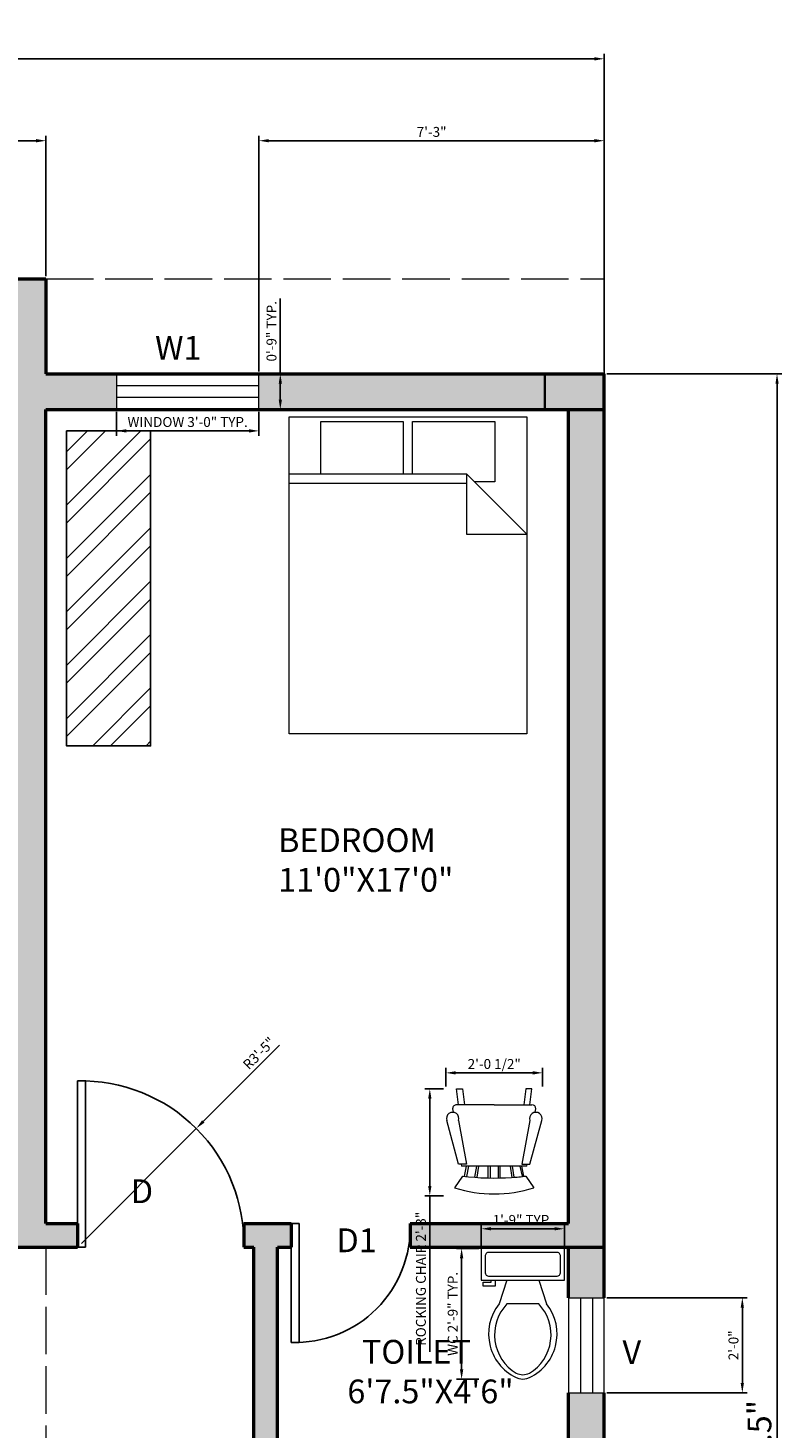
# Model space of a CAD drawing. Units: inches. Extents: x 5703 to 6226, y 10088 to 10813.
# Tile 5 of 5: x 6036 to 6226, y 10460 to 10813. Entities that reach past the tile are written whole.
import ezdxf

# ---------------------------------------------------------------- set-up
doc = ezdxf.new("R2010")
doc.units = ezdxf.units.IN
doc.linetypes.add('ACAD_ISO02W100', pattern=[15, 12, -3])
for name, color, linetype, lineweight in [('A-ANNO-DIMS', 2, 'Continuous', 18), ('A-ANNO-TEXT', 7, 'Continuous', 18), ('A-AREA-IDEN', 7, 'Continuous', 18), ('A-COLS', 7, 'Continuous', 35), ('A-COLS-PATT', 7, 'Continuous', 13), ('A-DOOR', 140, 'Continuous', 25), ('A-FLOR-CASE', 8, 'Continuous', 25), ('A-FLOR-CASE-PATT', 9, 'Continuous', 13), ('A-FLOR-FIXT', 8, 'Continuous', 18), ('A-FURN', 8, 'Continuous', 18), ('A-WALL', 7, 'Continuous', 50), ('A-WALL-PATT', 9, 'Continuous', 13)]:
    doc.layers.add(name, color=color, linetype=linetype, lineweight=lineweight)
for name, color, linetype, lineweight, true_color in [('A-GLAZ', 112, 'Continuous', 18, 0x1ce368), ('A-ROOF-OVHD', 30, 'ACAD_ISO02W100', 18, 0xf8991e), ('A-WALL-OVHD', 30, 'ACAD_ISO02W100', 18, 0xf8991e)]:
    doc.layers.add(name, color=color, linetype=linetype, lineweight=lineweight, true_color=true_color)
doc.styles.get("Standard").update_dxf_attribs({"font": 'arial.ttf'})
doc.dimstyles.new('ISO-25', dxfattribs={"dimtxt": 2.5, "dimasz": 2.5, "dimexe": 1.25, "dimexo": 0.625, "dimtad": 1, "dimlunit": 3, "dimtxsty": 'Standard', "dimcen": 2.5, "dimadec": 0, "dimazin": 0, "dimtfac": 1, "dimtmove": 0, "dimatfit": 3, "dimfxl": 1, "dimarcsym": 0})

# ---------------------------------------------------------------- blocks, each defined once
blk = doc.blocks.new('*D10')
at = {"layer": 'A-ANNO-DIMS', "color": 0, "lineweight": -2, "transparency": 16777216}
for p, q in [((5772.18, 10726.21), (5772.18, 10806.65)), ((5774.68, 10805.4), (6178.68, 10805.4)), ((6181.18, 10726.49), (6181.18, 10806.65))]:
    blk.add_line(p, q, dxfattribs=at)
at = {"layer": 'A-ANNO-DIMS', "color": 0, "transparency": 16777216}
for points in [[(5774.68, 10805.81), (5774.68, 10804.98), (5772.18, 10805.4)], [(6178.68, 10805.81), (6178.68, 10804.98), (6181.18, 10805.4)]]:
    blk.add_solid(points, dxfattribs=at)
at = {"layer": 'Defpoints', "color": 0, "transparency": 16777216}
for p in [(6181.18, 10805.4), (5772.18, 10725.59), (6181.18, 10725.87)]:
    blk.add_point(p, dxfattribs=at)
at = {"layer": 'A-ANNO-DIMS', "color": 0, "transparency": 16777216, "insert": (5976.68, 10809.09), "char_height": 6, "attachment_point": 5}
blk.add_mtext('34\'-0.99"', dxfattribs=at)
blk = doc.blocks.new('*D11')
at = {"layer": 'A-ANNO-DIMS', "color": 0, "lineweight": -2, "transparency": 16777216}
for p, q in [((6181.8, 10725.87), (6226.04, 10725.87)), ((6224.79, 10723.37), (6224.79, 10180.87)), ((6181.8, 10178.37), (6226.04, 10178.37))]:
    blk.add_line(p, q, dxfattribs=at)
at = {"layer": 'A-ANNO-DIMS', "color": 0, "transparency": 16777216}
for points in [[(6224.38, 10723.37), (6225.21, 10723.37), (6224.79, 10725.87)], [(6224.38, 10180.87), (6225.21, 10180.87), (6224.79, 10178.37)]]:
    blk.add_solid(points, dxfattribs=at)
at = {"layer": 'Defpoints', "color": 0, "transparency": 16777216}
for p in [(6181.18, 10725.87), (6181.18, 10178.37), (6224.79, 10178.37)]:
    blk.add_point(p, dxfattribs=at)
at = {"layer": 'A-ANNO-DIMS', "color": 0, "transparency": 16777216, "insert": (6221.12, 10452.12), "char_height": 6, "width": 12.5074, "attachment_point": 5, "rotation": 90}
blk.add_mtext('45\'-7.5"', dxfattribs=at)
blk = doc.blocks.new('Bed - Queen')
for p, q in [((0, -80.00003), (0, 0)), ((0, 0), (59.99999, 0)), ((59.99999, 0), (59.99999, -80.00003)), ((7.99999, -1.2), (28.79998, -1.2)), ((7.99999, -14.4), (7.99999, -1.2)), ((28.79998, -1.2), (28.79998, -14.4)), ((31.19999, -1.2), (51.99999, -1.2)), ((31.19999, -14.4), (31.19999, -1.2)), ((51.99999, -1.2), (51.99999, -16.4)), ((0, -14.4), (44.8, -14.4)), ((44.8, -16.8), (0, -16.8)), ((59.99999, -29.6), (44.8, -14.4)), ((44.8, -14.4), (44.8, -29.6)), ((51.99999, -16.4), (46.79936, -16.4)), ((44.8, -29.6), (59.99999, -29.6)), ((59.99999, -80.00003), (0, -80.00003))]:
    blk.add_line(p, q)
blk = doc.blocks.new('Toilet - top')
for p, q in [((9.5, -6), (9.5, -2)), ((-10, -8.5), (-8, -8.5)), ((-10, -9.5), (-10, -8.5)), ((-7, -9.5), (-10, -9.5)), ((-8, -8.5), (-8, -8)), ((-7, -8), (-7, -9.5)), ((-4, -8), (-6, -14)), ((4, -8), (6, -14)), ((4, -14), (-4, -14))]:
    blk.add_line(p, q)
blk.add_lwpolyline([(10.5, -8), (10.5, 0), (-10.5, 0), (-10.5, -8)], close=True)
for points in [[(-9.5, -2), (-9.5, -6)], [(8.5, -1), (-8.5, -1)], [(-8.5, -7), (8.5, -7)]]:
    blk.add_lwpolyline(points)
for centre, radius, start, end in [((-8.62, -1.88), 0.884, 81.8699, 188.1301), ((8.62, -1.88), 0.884, 351.8699, 98.1301), ((-8.62, -6.12), 0.884, 171.8699, 278.1301), ((8.62, -6.12), 0.884, 261.8699, 8.1301), ((3.52, -21.58), 12.17, 141.4691, 247.9714), ((4.2, -21.82), 11.33, 136.3677, 238.9468), ((-3.52, -21.58), 12.17, 292.0284, 38.5307), ((-4.2, -21.82), 11.33, 301.053, 43.6321), ((0, -27.88), 4, 245.7318, 294.2682), ((0, -29), 4, 254.8605, 285.1395)]:
    blk.add_arc(centre, radius, start, end)
blk = doc.blocks.new('Chair - Rocking')
for p, q in [((-8, -4.5), (-10, -1.5)), ((8, -4.5), (10, -1.5)), ((-8.23428, -6.99939), (-8.3093, -7.47958)), ((-8.23041, -7), (8.23915, -7)), ((-7.5, -4.5), (-7, -7)), ((-6.5, -7), (-7.02225, -4.43)), ((-4.5, -7), (-4.96674, -4.19951)), ((-4, -7), (-4.40532, -4.16272)), ((-1.5, -4.05012), (-1.5, -7)), ((-1, -7), (-1, -4.05012)), ((1, -7), (1, -4.04655)), ((1.5, -4.05012), (1.5, -7)), ((4, -7), (4.40187, -4.18694)), ((4.5, -7), (4.96761, -4.19437)), ((6.5, -7), (7, -4.4057)), ((7.5, -4.5), (7, -7)), ((8.31071, -7.48854), (8.23449, -7.00073)), ((-9, -7.5), (-12, -18.49999)), ((-7, -7.5), (-9, -7.5)), ((-9, -18.49999), (-7, -7.5)), ((7, -7.5), (9, -7.5)), ((9, -18.49999), (7, -7.5)), ((9, -7.5), (12, -18.49999)), ((-10.36644, -20.64523), (-10.5, -21.49999)), ((10.5, -21.49999), (10.3575, -20.58798)), ((-9, -22.49999), (-9.5, -26.49999)), ((0, -22.49999), (-9.5, -22.49999)), ((-8, -26.49999), (-7.5, -22.49999)), ((0, -22.49999), (9.5, -22.49999)), ((8, -26.49999), (7.5, -22.49999)), ((9, -22.49999), (9.5, -26.49999)), ((-9.5, -26.49999), (-8, -26.49999)), ((9.5, -26.49999), (8, -26.49999))]:
    blk.add_line(p, q)
for centre, radius, start, end in [((0, -34.08333), 34.08333, 72.93847, 107.0615), ((0, -68.25004), 64.25, 93.92211, 97.15267), ((0, -68.25004), 64.25, 82.84733, 93.92211), ((-10.5, -18.99999), 1.58114, 161.5651, 18.43495), ((10.5, -18.99999), 1.58114, 161.5651, 18.43495), ((-9.5, -21.49999), 1, 180, 270), ((9.5, -21.49999), 1, 270, 0)]:
    blk.add_arc(centre, radius, start, end)
blk = doc.blocks.new('WIN-36x9')
for p, q in [((0, 9), (0, 0)), ((36, 9), (0, 9)), ((36, 0), (36, 9)), ((36, 6), (0, 6)), ((36, 3), (0, 3)), ((0, 0), (36, 0))]:
    blk.add_line(p, q)
blk = doc.blocks.new('DOOR-SWING-30')
for p, q in [((0, 30.02), (0, 0.02)), ((2, 30.02), (0, 30.02)), ((2, 0.02), (2, 30.02)), ((0, 0.02), (2, 0.02))]:
    blk.add_line(p, q)
blk.add_arc((1, 29.02), 29.02, 268.0251, 1.9749)
blk = doc.blocks.new('*D20')
at = {"layer": 'A-ANNO-DIMS', "color": 0, "lineweight": -2, "transparency": 16777216}
for p, q in [((6149.48, 10505.1), (6143.9, 10505.1)), ((6145.15, 10474.55), (6145.15, 10502.6)), ((6149.48, 10472.05), (6143.9, 10472.05))]:
    blk.add_line(p, q, dxfattribs=at)
at = {"layer": 'A-ANNO-DIMS', "color": 0, "transparency": 16777216}
for points in [[(6144.73, 10502.6), (6145.57, 10502.6), (6145.15, 10505.1)], [(6144.73, 10474.55), (6145.57, 10474.55), (6145.15, 10472.05)]]:
    blk.add_solid(points, dxfattribs=at)
at = {"layer": 'Defpoints', "color": 0, "transparency": 16777216}
for p in [(6145.15, 10505.1), (6150.11, 10505.1), (6150.11, 10472.05)]:
    blk.add_point(p, dxfattribs=at)
at = {"layer": 'A-ANNO-DIMS', "color": 0, "transparency": 16777216, "insert": (6143.23, 10488.57), "char_height": 2.5, "attachment_point": 5, "rotation": 90}
blk.add_mtext('WC 2\'-9" TYP.', dxfattribs=at)
blk = doc.blocks.new('*D21')
at = {"layer": 'A-ANNO-DIMS', "color": 0, "lineweight": -2, "transparency": 16777216}
for p, q in [((6150.11, 10505.72), (6150.11, 10511.3)), ((6171.11, 10505.72), (6171.11, 10511.3)), ((6152.61, 10510.05), (6168.61, 10510.05))]:
    blk.add_line(p, q, dxfattribs=at)
at = {"layer": 'A-ANNO-DIMS', "color": 0, "transparency": 16777216}
for points in [[(6152.61, 10510.47), (6152.61, 10509.64), (6150.11, 10510.05)], [(6168.61, 10510.47), (6168.61, 10509.64), (6171.11, 10510.05)]]:
    blk.add_solid(points, dxfattribs=at)
at = {"layer": 'Defpoints', "color": 0, "transparency": 16777216}
for p in [(6171.11, 10510.05), (6150.11, 10505.1), (6171.11, 10505.1)]:
    blk.add_point(p, dxfattribs=at)
at = {"layer": 'A-ANNO-DIMS', "color": 0, "transparency": 16777216, "insert": (6160.61, 10511.96), "char_height": 2.5, "attachment_point": 5}
blk.add_mtext('1\'-9" TYP.', dxfattribs=at)
blk = doc.blocks.new('*D22')
at = {"layer": 'A-ANNO-DIMS', "color": 0, "lineweight": -2, "transparency": 16777216}
for p, q in [((6057.98, 10716.24), (6057.98, 10710.22)), ((6093.98, 10716.24), (6093.98, 10710.22)), ((6060.48, 10711.47), (6091.48, 10711.47))]:
    blk.add_line(p, q, dxfattribs=at)
at = {"layer": 'A-ANNO-DIMS', "color": 0, "transparency": 16777216}
for points in [[(6060.48, 10711.89), (6060.48, 10711.05), (6057.98, 10711.47)], [(6091.48, 10711.89), (6091.48, 10711.05), (6093.98, 10711.47)]]:
    blk.add_solid(points, dxfattribs=at)
at = {"layer": 'Defpoints', "color": 0, "transparency": 16777216}
for p in [(6057.98, 10716.87), (6093.98, 10716.87), (6093.98, 10711.47)]:
    blk.add_point(p, dxfattribs=at)
at = {"layer": 'A-ANNO-DIMS', "color": 0, "transparency": 16777216, "insert": (6075.98, 10713.39), "char_height": 2.5, "attachment_point": 5}
blk.add_mtext('WINDOW 3\'-0" TYP.', dxfattribs=at)
blk = doc.blocks.new('*D23')
at = {"layer": 'A-ANNO-DIMS', "color": 0, "lineweight": -2, "transparency": 16777216}
for p, q in [((6099.38, 10725.87), (6099.38, 10744.86)), ((6094.61, 10725.87), (6100.63, 10725.87)), ((6099.38, 10719.37), (6099.38, 10723.37)), ((6094.61, 10716.87), (6100.63, 10716.87))]:
    blk.add_line(p, q, dxfattribs=at)
at = {"layer": 'A-ANNO-DIMS', "color": 0, "transparency": 16777216}
for points in [[(6098.97, 10723.37), (6099.8, 10723.37), (6099.38, 10725.87)], [(6098.97, 10719.37), (6099.8, 10719.37), (6099.38, 10716.87)]]:
    blk.add_solid(points, dxfattribs=at)
at = {"layer": 'Defpoints', "color": 0, "transparency": 16777216}
for p in [(6093.98, 10725.87), (6099.38, 10725.87), (6093.98, 10716.87)]:
    blk.add_point(p, dxfattribs=at)
at = {"layer": 'A-ANNO-DIMS', "color": 0, "transparency": 16777216, "insert": (6097.48, 10736.61), "char_height": 2.5, "attachment_point": 5, "rotation": 90}
blk.add_mtext('0\'-9" TYP.', dxfattribs=at)
blk = doc.blocks.new('*D34')
at = {"layer": 'A-ANNO-DIMS', "color": 0, "lineweight": -2, "transparency": 16777216}
for p, q in [((6140.55, 10545.36), (6135.87, 10545.36)), ((6137.12, 10542.86), (6137.12, 10520.86)), ((6140.55, 10518.36), (6135.87, 10518.36)), ((6137.12, 10518.36), (6137.12, 10478.99))]:
    blk.add_line(p, q, dxfattribs=at)
at = {"layer": 'A-ANNO-DIMS', "color": 0, "transparency": 16777216}
for points in [[(6136.71, 10542.86), (6137.54, 10542.86), (6137.12, 10545.36)], [(6136.71, 10520.86), (6137.54, 10520.86), (6137.12, 10518.36)]]:
    blk.add_solid(points, dxfattribs=at)
at = {"layer": 'Defpoints', "color": 0, "transparency": 16777216}
for p in [(6141.17, 10545.36), (6137.12, 10518.36), (6141.17, 10518.36)]:
    blk.add_point(p, dxfattribs=at)
at = {"layer": 'A-ANNO-DIMS', "color": 0, "transparency": 16777216, "insert": (6135.2, 10497.42), "char_height": 2.5, "attachment_point": 5, "rotation": 90}
blk.add_mtext('ROCKING CHAIR 2\'-3"', dxfattribs=at)
blk = doc.blocks.new('*D35')
at = {"layer": 'A-ANNO-DIMS', "color": 0, "lineweight": -2, "transparency": 16777216}
for p, q in [((6141.17, 10545.98), (6141.17, 10550.66)), ((6165.61, 10545.98), (6165.61, 10550.66)), ((6163.11, 10549.41), (6143.67, 10549.41))]:
    blk.add_line(p, q, dxfattribs=at)
at = {"layer": 'A-ANNO-DIMS', "color": 0, "transparency": 16777216}
for points in [[(6143.67, 10549.83), (6143.67, 10548.99), (6141.17, 10549.41)], [(6163.11, 10549.83), (6163.11, 10548.99), (6165.61, 10549.41)]]:
    blk.add_solid(points, dxfattribs=at)
at = {"layer": 'Defpoints', "color": 0, "transparency": 16777216}
for p in [(6141.17, 10549.41), (6141.17, 10545.36), (6165.61, 10545.36)]:
    blk.add_point(p, dxfattribs=at)
at = {"layer": 'A-ANNO-DIMS', "color": 0, "transparency": 16777216, "insert": (6153.39, 10551.33), "char_height": 2.5, "attachment_point": 5}
blk.add_mtext('2\'-0 1/2"', dxfattribs=at)
blk = doc.blocks.new('*D44')
at = {"layer": 'A-ANNO-DIMS', "color": 0, "lineweight": -2, "transparency": 16777216}
for p, q in [((5902.18, 10750.49), (5902.18, 10785.97)), ((5904.68, 10784.72), (6037.68, 10784.72)), ((6040.18, 10750.49), (6040.18, 10785.97))]:
    blk.add_line(p, q, dxfattribs=at)
at = {"layer": 'A-ANNO-DIMS', "color": 0, "transparency": 16777216}
for points in [[(5904.68, 10785.14), (5904.68, 10784.3), (5902.18, 10784.72)], [(6037.68, 10785.14), (6037.68, 10784.3), (6040.18, 10784.72)]]:
    blk.add_solid(points, dxfattribs=at)
at = {"layer": 'Defpoints', "color": 0, "transparency": 16777216}
for p in [(6040.18, 10784.72), (5902.18, 10749.87), (6040.18, 10749.87)]:
    blk.add_point(p, dxfattribs=at)
at = {"layer": 'A-ANNO-DIMS', "color": 0, "transparency": 16777216, "insert": (5971.18, 10786.62), "char_height": 2.5, "attachment_point": 5}
blk.add_mtext('11\'-6"', dxfattribs=at)
blk = doc.blocks.new('*D54')
at = {"layer": 'A-ANNO-DIMS', "color": 0, "lineweight": -2, "transparency": 16777216}
for p, q in [((6181.8, 10492.63), (6217.28, 10492.63)), ((6216.03, 10471.13), (6216.03, 10490.13)), ((6181.8, 10468.63), (6217.28, 10468.63))]:
    blk.add_line(p, q, dxfattribs=at)
at = {"layer": 'A-ANNO-DIMS', "color": 0, "transparency": 16777216}
for points in [[(6215.61, 10490.13), (6216.44, 10490.13), (6216.03, 10492.63)], [(6215.61, 10471.13), (6216.44, 10471.13), (6216.03, 10468.63)]]:
    blk.add_solid(points, dxfattribs=at)
at = {"layer": 'Defpoints', "color": 0, "transparency": 16777216}
for p in [(6181.18, 10492.63), (6216.03, 10492.63), (6181.18, 10468.63)]:
    blk.add_point(p, dxfattribs=at)
at = {"layer": 'A-ANNO-DIMS', "color": 0, "transparency": 16777216, "insert": (6214.12, 10480.63), "char_height": 2.5, "attachment_point": 5, "rotation": 90}
blk.add_mtext('2\'-0"', dxfattribs=at)
blk = doc.blocks.new('*D57')
at = {"layer": 'A-ANNO-DIMS', "color": 0, "lineweight": -2, "transparency": 16777216}
for p, q in [((6093.98, 10726.49), (6093.98, 10785.97)), ((6096.48, 10784.72), (6178.68, 10784.72)), ((6181.18, 10726.49), (6181.18, 10785.97))]:
    blk.add_line(p, q, dxfattribs=at)
at = {"layer": 'A-ANNO-DIMS', "color": 0, "transparency": 16777216}
for points in [[(6096.48, 10785.14), (6096.48, 10784.3), (6093.98, 10784.72)], [(6178.68, 10785.14), (6178.68, 10784.3), (6181.18, 10784.72)]]:
    blk.add_solid(points, dxfattribs=at)
at = {"layer": 'Defpoints', "color": 0, "transparency": 16777216}
for p in [(6181.18, 10784.72), (6093.98, 10725.87), (6181.18, 10725.87)]:
    blk.add_point(p, dxfattribs=at)
at = {"layer": 'A-ANNO-DIMS', "color": 0, "transparency": 16777216, "insert": (6137.58, 10786.62), "char_height": 2.5, "attachment_point": 5}
blk.add_mtext('7\'-3"', dxfattribs=at)
blk = doc.blocks.new('*D59')
at = {"layer": 'A-ANNO-DIMS', "color": 0, "lineweight": -2, "transparency": 16777216}
for p, q in [((6099.2, 10556.41), (6079.93, 10537.14)), ((6049.16, 10506.37), (6078.16, 10535.37))]:
    blk.add_line(p, q, dxfattribs=at)
at = {"layer": 'A-ANNO-DIMS', "color": 0, "transparency": 16777216}
blk.add_solid([(6079.63, 10537.43), (6080.22, 10536.84), (6078.16, 10535.37)], dxfattribs=at)
at = {"layer": 'Defpoints', "color": 0, "transparency": 16777216}
for p in [(6078.16, 10535.37), (6049.16, 10506.37)]:
    blk.add_point(p, dxfattribs=at)
at = {"layer": 'A-ANNO-DIMS', "color": 0, "transparency": 16777216, "insert": (6094.22, 10554.11), "char_height": 2.5, "attachment_point": 5, "rotation": 45.0005}
blk.add_mtext('R3\'-5"', dxfattribs=at)

msp = doc.modelspace()

# ---------------------------------------------------------------- hatches: boundary and pattern name
at = {"layer": 'A-COLS-PATT'}
h = msp.add_hatch(color=256, dxfattribs=at)
h.dxf.hatch_style = 1
h.paths.add_polyline_path([(5788.176, 10725.869), (5773.176, 10725.869), (5773.176, 10716.869), (5788.176, 10716.869)])
h.paths.add_polyline_path([(5782.176, 10516.684), (5773.176, 10516.684), (5773.176, 10497.849), (5782.176, 10497.849)])
h.paths.add_polyline_path([(5782.176, 10319.369), (5773.176, 10319.369), (5773.176, 10304.369), (5782.176, 10304.369)])
h.paths.add_polyline_path([(5960.955, 10313.369), (5953.525, 10313.369), (5953.525, 10304.369), (5960.955, 10304.369)])
h.paths.add_polyline_path([(6040.176, 10314.869), (6031.176, 10314.869), (6031.176, 10304.369), (6040.176, 10304.369)])
h.paths.add_polyline_path([(6181.176, 10198.545), (6172.176, 10198.545), (6172.176, 10178.369), (6181.176, 10178.369)])
h.paths.add_polyline_path([(6181.176, 10505.369), (6172.176, 10505.369), (6172.176, 10492.633), (6181.176, 10492.633)])
h.paths.add_polyline_path([(6181.176, 10725.869), (6166.176, 10725.869), (6166.176, 10716.869), (6181.176, 10716.869)])
at = {"layer": 'A-FLOR-CASE-PATT'}
h = msp.add_hatch(dxfattribs=at)
h.set_pattern_fill('ANSI32', color=256)
h.paths.add_polyline_path([(6066.642, 10711.473), (6045.414, 10711.473), (6045.414, 10631.936), (6066.642, 10631.936)])
at = {"layer": 'A-WALL-PATT'}
h = msp.add_hatch(color=256, dxfattribs=at)
h.dxf.hatch_style = 1
h.paths.add_polyline_path([(6057.982, 10725.869), (6040.176, 10725.869), (6040.176, 10749.869), (5999.271, 10749.869), (5999.271, 10740.869), (6031.176, 10740.869), (6031.176, 10716.869), (6031.176, 10511.369), (6013.525, 10511.369), (6013.525, 10505.369), (6048.161, 10505.369), (6048.161, 10511.369), (6040.176, 10511.369), (6040.176, 10716.869), (6057.982, 10716.869)])
h.paths.add_polyline_path([(6166.176, 10725.869), (6093.982, 10725.869), (6093.982, 10716.869), (6166.176, 10716.869)])
h.paths.add_polyline_path([(6181.176, 10716.869), (6172.176, 10716.869), (6172.176, 10511.369), (6132.161, 10511.369, -0.0172363), (6132.161, 10509.369), (6132.161, 10505.369), (6181.176, 10505.369)])
h.paths.add_polyline_path([(6181.176, 10468.633), (6172.176, 10468.633), (6172.176, 10451.369), (6098.676, 10451.369), (6098.676, 10505.369), (6102.161, 10505.369), (6102.161, 10511.369), (6090.161, 10511.369), (6090.161, 10507.369, -0.0121933), (6090.161, 10505.369), (6092.676, 10505.369), (6092.676, 10451.369), (6085.668, 10451.369), (6085.668, 10445.369), (6092.676, 10445.369), (6172.176, 10445.369), (6172.176, 10342.529), (6181.176, 10342.529)])
h.paths.add_polyline_path([(6181.176, 10282.529), (6172.176, 10282.529), (6172.176, 10253.369), (6092.676, 10253.369), (6092.676, 10247.369), (6094.176, 10247.369), (6094.176, 10238.954), (6100.176, 10238.954), (6100.176, 10247.369), (6172.176, 10247.369), (6172.176, 10234.545), (6181.176, 10234.545)])
h.paths.add_polyline_path([(6172.176, 10187.369), (6100.176, 10187.369), (6100.176, 10220.954), (6096.176, 10220.954, -0.0293864), (6094.176, 10220.954), (6094.176, 10178.369), (6172.176, 10178.369)])
h.paths.add_polyline_path([(6050.745, 10187.369), (6040.176, 10187.369), (6040.176, 10178.369), (6050.745, 10178.369)])
h.paths.add_polyline_path([(6040.176, 10187.369), (6031.176, 10187.369), (6031.176, 10178.369), (6040.176, 10178.369)])
h.paths.add_polyline_path([(6040.176, 10304.369), (6031.176, 10304.369), (6031.176, 10187.369), (6040.176, 10187.369)])
h.paths.add_polyline_path([(6040.176, 10393.328), (6031.176, 10393.328), (6031.176, 10314.869), (6040.176, 10314.869)])
h.paths.add_polyline_path([(6040.176, 10445.369), (6046.458, 10445.369), (6046.458, 10451.369), (6031.176, 10451.369), (6031.176, 10408.328), (6040.176, 10408.328)])
h.paths.add_polyline_path([(5911.176, 10584.869), (5845.666, 10584.869, -0.0172363), (5845.666, 10582.869), (5845.666, 10578.869), (5902.176, 10578.869), (5902.176, 10505.369), (5953.525, 10505.369), (5953.525, 10511.369), (5911.176, 10511.369)])
h.paths.add_polyline_path([(5902.176, 10511.369), (5782.176, 10511.369), (5782.176, 10505.369), (5902.176, 10505.369)])
h.paths.add_polyline_path([(5782.176, 10578.869), (5815.666, 10578.869), (5815.666, 10584.869), (5773.176, 10584.869), (5773.176, 10516.684), (5782.176, 10516.684)])
h.paths.add_polyline_path([(5782.176, 10497.849), (5773.176, 10497.849), (5773.176, 10438.429), (5782.176, 10438.429)])
h.paths.add_polyline_path([(5782.176, 10378.429), (5773.176, 10378.429), (5773.176, 10319.369), (5782.176, 10319.369)])
h.paths.add_polyline_path([(5824.846, 10313.369), (5782.176, 10313.369), (5782.176, 10304.369), (5824.846, 10304.369)])
h.paths.add_polyline_path([(5953.525, 10313.369), (5872.846, 10313.369), (5872.846, 10304.369), (5953.525, 10304.369)])

# ---------------------------------------------------------------- linework, layer by layer
at = {"layer": 'A-COLS'}
for p, q in [((6181.176, 10725.869), (6166.176, 10725.869)), ((6166.176, 10725.869), (6166.176, 10716.869))]:
    msp.add_line(p, q, dxfattribs=at)
at = {"layer": 'A-DOOR'}
for p, q in [((6048.161, 10505.369), (6048.161, 10547.369)), ((6048.161, 10547.369), (6050.161, 10547.369)), ((6050.161, 10547.369), (6050.161, 10505.369)), ((6102.161, 10511.369), (6102.161, 10511.369)), ((6050.161, 10505.369), (6048.161, 10505.369))]:
    msp.add_line(p, q, dxfattribs=at)
msp.add_arc((6049.161, 10506.369), 41.012, 358.60282, 91.39718, dxfattribs=at)
at = {"layer": 'A-FLOR-CASE'}
msp.add_lwpolyline([(6045.414, 10711.473), (6066.642, 10711.473), (6066.642, 10631.936), (6045.414, 10631.936)], close=True, dxfattribs=at)
at = {"layer": 'A-GLAZ'}
for p, q in [((6172.176, 10492.633), (6181.176, 10492.633)), ((6172.176, 10492.633), (6172.176, 10468.633)), ((6175.176, 10492.633), (6175.176, 10468.633)), ((6178.176, 10492.633), (6178.176, 10468.633)), ((6181.176, 10468.633), (6181.176, 10492.633)), ((6172.176, 10468.633), (6181.176, 10468.633)), ((6172.176, 10468.633), (6181.176, 10468.633))]:
    msp.add_line(p, q, dxfattribs=at)
at = {"layer": 'A-ROOF-OVHD'}
for p, q in [((6040.176, 10749.869), (6181.176, 10749.869)), ((6181.176, 10749.869), (6181.176, 10725.869))]:
    msp.add_line(p, q, dxfattribs=at)
at = {"layer": 'A-WALL'}
for p, q in [((5902.176, 10749.869), (6040.176, 10749.869)), ((6040.176, 10749.869), (6040.176, 10725.869)), ((6040.176, 10725.869), (6181.176, 10725.869)), ((6181.176, 10492.633), (6181.176, 10725.869)), ((6040.176, 10716.869), (6181.176, 10716.869)), ((6040.176, 10511.369), (6040.176, 10716.869)), ((6172.176, 10511.369), (6172.176, 10716.869)), ((6040.176, 10511.369), (6048.161, 10511.369)), ((6048.161, 10511.369), (6048.161, 10505.369)), ((6090.161, 10511.369), (6090.161, 10505.369)), ((6090.161, 10511.369), (6102.161, 10511.369)), ((6102.161, 10511.369), (6102.161, 10505.369)), ((6132.161, 10511.369), (6132.161, 10505.369)), ((6132.161, 10511.369), (6172.176, 10511.369)), ((6013.525, 10505.369), (6048.161, 10505.369)), ((6090.161, 10505.369), (6092.676, 10505.369)), ((6092.676, 10451.369), (6092.676, 10505.369)), ((6098.676, 10451.369), (6098.676, 10505.369)), ((6098.676, 10505.369), (6102.161, 10505.369)), ((6132.161, 10505.369), (6181.176, 10505.369)), ((6172.176, 10492.633), (6172.176, 10505.369)), ((6172.176, 10451.369), (6172.176, 10468.633)), ((6181.176, 10178.369), (6181.176, 10468.633))]:
    msp.add_line(p, q, dxfattribs=at)
at = {"layer": 'A-WALL-OVHD'}
msp.add_line((6040.176, 10505.369), (6040.176, 10451.369), dxfattribs=at)

# ---------------------------------------------------------------- block references
at = {"layer": 'A-DOOR'}
msp.add_blockref('DOOR-SWING-30', (6102.162, 10481.352), dxfattribs=at)
at = {"layer": 'A-FLOR-FIXT'}
msp.add_blockref('Toilet - top', (6160.608, 10505.098), dxfattribs=at)
at = {"layer": 'A-FURN'}
msp.add_blockref('Bed - Queen', (6101.582, 10715.028), dxfattribs=at)
at = {"layer": 'A-FURN', "rotation": 180}
msp.add_blockref('Chair - Rocking', (6153.391, 10518.859), dxfattribs=at)
at = {"layer": 'A-GLAZ'}
msp.add_blockref('WIN-36x9', (6057.982, 10716.869), dxfattribs=at)

# ---------------------------------------------------------------- texts
at = {"layer": 'A-ANNO-TEXT', "char_height": 6, "attachment_point": 1}
for s, insert in [(' W1', (6065.919, 10735.444)), (' D', (6059.792, 10522.524)), (' D1', (6111.724, 10510.142)), (' V', (6183.93, 10481.878))]:
    msp.add_mtext_dynamic_manual_height_columns(s, width=71.13425, gutter_width=12.5, heights=[0], dxfattribs=dict(at, insert=insert))
at = {"layer": 'A-AREA-IDEN', "char_height": 6, "attachment_point": 1}
for s, insert in [(' BEDROOM\\P 11\'0"X17\'0"', (6096.997, 10611.145)), ('   TOILET\\P 6\'7.5"X4\'6"', (6114.472, 10481.991))]:
    msp.add_mtext_dynamic_manual_height_columns(s, width=71.13425, gutter_width=12.5, heights=[0], dxfattribs=dict(at, insert=insert))

# ---------------------------------------------------------------- dimensions: what is measured, and where the dimension line sits
at = {"layer": 'A-ANNO-DIMS'}
for base, p1, p2, override, picture, middle in [((6181.176, 10805.396), (5772.182, 10725.59), (6181.176, 10725.869), {"dimtxt": 6, "dimclrd": 0, "dimclre": 0, "dimclrt": 0}, '*D10', (5976.679, 10809.086)), ((6040.176, 10784.719), (5902.176, 10749.869), (6040.176, 10749.869), {"dimdec": 1, "dimlfac": 1, "dimrnd": 0, "dimzin": 1, "dimdsep": 46, "dimlunit": 4, "dimfrac": 2}, '*D44', (5971.176, 10786.62)), ((6181.176, 10784.719), (6093.982, 10725.869), (6181.176, 10725.869), {"dimdec": 1, "dimlfac": 1, "dimrnd": 0, "dimzin": 1, "dimdsep": 46, "dimlunit": 4, "dimfrac": 2}, '*D57', (6137.579, 10786.621))]:
    dim = msp.add_linear_dim(base=base, p1=p1, p2=p2, dimstyle='ISO-25', override=override, dxfattribs=at)
    dim.commit()
    dim.dimension.update_dxf_attribs({"geometry": picture, "text_midpoint": middle})
for base, p1, p2, angle, text, picture, middle in [((6099.382, 10725.869), (6093.982, 10716.869), (6093.982, 10725.869), 90, '<> TYP.', '*D23', (6097.48, 10736.613)), ((6137.124, 10518.359), (6141.174, 10545.359), (6141.174, 10518.359), 270, 'ROCKING CHAIR <>', '*D34', (6135.205, 10497.423)), ((6145.151, 10505.098), (6150.108, 10472.052), (6150.108, 10505.098), 90, 'WC <> TYP.', '*D20', (6143.233, 10488.575))]:
    dim = msp.add_linear_dim(base=base, p1=p1, p2=p2, angle=angle, text=text, dimstyle='ISO-25', override={"dimdec": 1, "dimlfac": 1, "dimrnd": 0, "dimzin": 1, "dimdsep": 46, "dimlunit": 4, "dimfrac": 2}, dxfattribs=at)
    dim.commit()
    dim.dimension.update_dxf_attribs({"geometry": picture, "text_midpoint": middle})
for base, p1, p2, angle, override, picture, middle in [((6224.795, 10178.369), (6181.176, 10725.869), (6181.176, 10178.369), 90, {"dimtxt": 6, "dimclrd": 0, "dimclre": 0, "dimclrt": 0}, '*D11', (6221.118, 10452.119)), ((6141.174, 10549.409), (6165.609, 10545.359), (6141.174, 10545.359), 180, {"dimdec": 1, "dimlfac": 1, "dimrnd": 0, "dimzin": 1, "dimdsep": 46, "dimlunit": 4, "dimfrac": 2}, '*D35', (6153.391, 10551.327)), ((6216.026, 10492.633), (6181.176, 10468.633), (6181.176, 10492.633), 90, {"dimdec": 1, "dimlfac": 1, "dimrnd": 0, "dimzin": 1, "dimdsep": 46, "dimlunit": 4, "dimfrac": 2}, '*D54', (6214.125, 10480.633))]:
    dim = msp.add_linear_dim(base=base, p1=p1, p2=p2, angle=angle, dimstyle='ISO-25', override=override, dxfattribs=at)
    dim.commit()
    dim.dimension.update_dxf_attribs({"geometry": picture, "text_midpoint": middle})
for base, p1, p2, text, picture, middle in [((6093.982, 10711.469), (6057.982, 10716.869), (6093.982, 10716.869), 'WINDOW <> TYP.', '*D22', (6075.982, 10713.388)), ((6171.108, 10510.055), (6150.108, 10505.098), (6171.108, 10505.098), '<> TYP.', '*D21', (6160.608, 10511.956))]:
    dim = msp.add_linear_dim(base=base, p1=p1, p2=p2, text=text, dimstyle='ISO-25', override={"dimdec": 1, "dimlfac": 1, "dimrnd": 0, "dimzin": 1, "dimdsep": 46, "dimlunit": 4, "dimfrac": 2}, dxfattribs=at)
    dim.commit()
    dim.dimension.update_dxf_attribs({"geometry": picture, "text_midpoint": middle})
dim = msp.add_radius_dim(center=(6049.161, 10506.369), mpoint=(6078.161, 10535.369), dimstyle='ISO-25', override={"dimdec": 1, "dimlfac": 1, "dimrnd": 0, "dimzin": 1, "dimdsep": 46, "dimlunit": 4, "dimfrac": 2}, dxfattribs=at)
dim.commit()
dim.dimension.update_dxf_attribs({"geometry": '*D59', "text_midpoint": (6095.561, 10552.769), "dimtype": 164})

doc.saveas('drawing.dxf')
